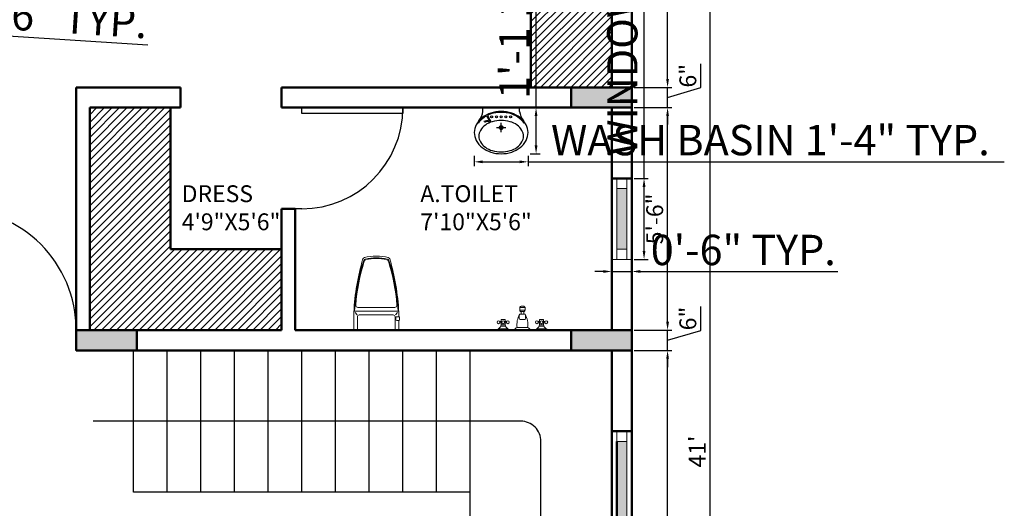
# Model space of a CAD drawing. Units: inches. Extents: x 3064 to 19385, y 846 to 15425.
# Tile 74 of 108: x 6629 to 6922, y 1725 to 1870. Entities that reach past the tile are written whole.
import ezdxf

# ---------------------------------------------------------------- set-up
doc = ezdxf.new("R2010")
doc.units = ezdxf.units.IN
for name, color, linetype, lineweight in [('A-ANNO-DIMS', 2, 'Continuous', 18), ('A-AREA-IDEN', 3, 'Continuous', 18), ('A-COLS', 1, 'Continuous', 35), ('A-DOOR', 3, 'Continuous', 25), ('A-FLOR-FIXT', 9, 'Continuous', 18), ('A-FLOR-STRS', 2, 'Continuous', 25), ('A-FURN-PATT', 252, 'Continuous', 13), ('A-GLAZ', 4, 'Continuous', 18), ('A-WALL', 7, 'Continuous', 50)]:
    doc.layers.add(name, color=color, linetype=linetype, lineweight=lineweight)
doc.layers.add('THIET-BI', color=21, linetype='Continuous')
doc.styles.get("Standard").update_dxf_attribs({"font": 'arial.ttf'})
doc.dimstyles.new('ISO-25', dxfattribs={"dimtxt": 9, "dimasz": 2.5, "dimexe": 1.25, "dimexo": 0.625, "dimtad": 1, "dimdec": 1, "dimlunit": 3, "dimtxsty": 'Standard', "dimcen": 2.5, "dimadec": 0, "dimazin": 0, "dimtfac": 1, "dimtdec": 1, "dimtmove": 0, "dimatfit": 3, "dimfxl": 1, "dimarcsym": 0})
pattern_1 = [(45, (2126.5405, 591.649), (-1.122532, 1.122532), [])]

# ---------------------------------------------------------------- blocks, each defined once
blk = doc.blocks.new('*U3')
for p, q in [((0, 0), (0, -6)), ((36, 0), (36, -6))]:
    blk.add_line(p, q)
blk.add_lwpolyline([(0, 0), (0, 36), (1.75, 36), (1.75, 0)], close=True)
blk.add_arc((0, 0), 36, 0, 90)
blk = doc.blocks.new('*U4')
for p, q in [((0, 0), (0, -6)), ((30, 0), (30, -6))]:
    blk.add_line(p, q)
blk.add_lwpolyline([(0, 0), (0, 30), (1.75, 30), (1.75, 0)], close=True)
blk.add_arc((0, 0), 30, 0, 90)
blk = doc.blocks.new('A$C430D11A0')
at = {"layer": 'THIET-BI'}
for p, q in [((90, 445), (90, 485)), ((475, 485), (90, 485)), ((475, 483), (90, 483)), ((475, 445), (475, 485)), ((129, 398), (158, 344)), ((138, 403), (176, 332)), ((282, 226), (282, 325)), ((233, 275), (332, 275))]:
    blk.add_line(p, q, dxfattribs=at)
for points in [[(565, 223, 0.121635), (545, 305, 0.10526), (482, 380, 0.088175), (393, 427, 0.079002), (282, 445, 0.079002), (172, 427, 0.088175), (83, 380, 0.10526), (20, 305, 0.121635), (0, 223, 0.121635), (20, 140, 0.10526), (83, 65, 0.088175), (172, 18, 0.079002), (282, 0, 0.079002), (393, 18, 0.088175), (482, 65, 0.10526), (545, 140, 0.121635)], [(517, 185, 0.134042), (501, 245, 0.106817), (449, 302, 0.082468), (376, 337, 0.070874), (282, 350, 0.070874), (189, 337, 0.082468), (116, 302, 0.106817), (64, 245, 0.134042), (47, 185, 0.134042), (64, 125, 0.106817), (116, 68, 0.082468), (189, 33, 0.070874), (282, 20, 0.070874), (376, 33, 0.082468), (449, 68, 0.106817), (501, 125, 0.134042)]]:
    blk.add_lwpolyline(points, format="xyb", close=True, dxfattribs=at)
for points in [[(523, 322, 0.07708), (476, 372, 0.088175), (390, 418, 0.079002), (282, 435, 0.079002), (175, 418, 0.035427), (138, 403, 0.07708)], [(129, 398, 0.043566), (89, 372, 0.07708), (42, 322, 0.041486)]]:
    blk.add_lwpolyline(points, format="xyb", dxfattribs=at)
for centre, radius in [((182, 388), 10.5), ((232, 388), 10.5), ((282, 388), 10.5), ((332, 388), 10.5), ((382, 388), 10.5), ((282, 275), 20), ((282, 275), 15)]:
    blk.add_circle(centre, radius, dxfattribs=at)
for centre, radius, start, end in [((-104, 469), 195, 320.8253, 352.9557), ((669, 469), 195, 187.0443, 219.1747), ((136, 285), 62.9, 69.643, 123.4774), ((136, 285), 52.9, 55.2455, 123.4774)]:
    blk.add_arc(centre, radius, start, end, dxfattribs=at)
blk = doc.blocks.new('WC-P05')
for p, q in [((-202, 532), (-202, 439)), ((-192, 542), (263, 542)), ((-163, 542), (-163, 401)), ((234, 542), (234, 401)), ((273, 532), (273, 352)), ((-210, 430), (-210, 409)), ((-201, 439), (-180, 439)), ((-171, 430), (-171, 409)), ((-202, 400), (-202, 352)), ((-201, 400), (-180, 400)), ((-192, 342), (263, 342)), ((-167, 379), (-188, 357)), ((-143, 381), (214, 381)), ((237, 379), (258, 357)), ((-159, 303), (229, 303))]:
    blk.add_line(p, q)
blk.add_lwpolyline([(-91, -222, 0.114547), (161, -222, 0.114547)], format="xyb")
for centre, radius, start, end in [((-192, 532), 10, 90, 180), ((263, 532), 10, 0, 90), ((-201, 430), 9, 90, 180), ((-180, 430), 9, 0, 90), ((-201, 409), 9, 180, 270), ((2309, 492), 2515, 183.2067, 196.1242), ((-192, 352), 10, 180, 270), ((1906, 447), 2103, 182.8743, 197.6554), ((-180, 409), 9, 270, 0), ((-143, 401), 20, 180, 270), ((-1836, 447), 2103, 342.3446, 357.1257), ((-2239, 492), 2515, 343.8727, 356.7933), ((214, 401), 20, 270, 0), ((263, 352), 10, 270, 0), ((-159, 280), 22.5, 90, 184.6246), ((1906, 447), 2095, 184.6245, 197.5277), ((-1836, 447), 2095, 342.464, 355.3754), ((229, 280), 22.5, 355.3754, 90), ((-86, -200), 22.5, 196.1242, 256.8994), ((-76, -184), 22.5, 197.6554, 257.5059), ((-70, -177), 22.5, 197.5277, 258.1005), ((35, 318), 536, 257.5059, 282.4941), ((36, 324), 535, 258.1005, 281.7373), ((140, -177), 22.5, 281.7373, 342.464), ((146, -184), 22.5, 282.4941, 342.3446), ((156, -200), 22.5, 283.0378, 343.8727)]:
    blk.add_arc(centre, radius, start, end)
blk = doc.blocks.new('Faucet - Bathroom front')
for p, q in [((-0.5, 4.25), (0.5, 4.25)), ((0.5, 3.75), (-0.5, 3.75)), ((-0.5, 3), (0.5, 3)), ((0.5, 2), (-0.5, 2)), ((-0.25, 3), (-0.25, 3.5)), ((0.25, 3.5), (0.25, 3)), ((-5, 0), (-2.25, 0)), ((-4.5087, 0.25), (-2.7408, 0.25)), ((-4, 1.625), (-4.25, 1.625)), ((-4, 1.375), (-4.25, 1.375)), ((-3.1442, 0.75), (-4.0979, 0.75)), ((-3.25, 1.625), (-3, 1.625)), ((-3.25, 1.375), (-3, 1.375)), ((-1.5, 0), (1.5, 0)), ((-1, 0.5), (1, 0.5)), ((2.25, 0), (5, 0)), ((2.7413, 0.25), (4.5092, 0.25)), ((3.25, 1.625), (3, 1.625)), ((3.25, 1.375), (3, 1.375)), ((4.1058, 0.75), (3.1521, 0.75)), ((4, 1.625), (4.25, 1.625)), ((4, 1.375), (4.25, 1.375))]:
    blk.add_line(p, q)
for points in [[(-0.5, 3.75), (-0.5, 4.25)], [(-0.25, 4.5), (0.25, 4.5)], [(0.5, 4.25), (0.5, 3.75)], [(0.25, 3.5), (-0.25, 3.5)]]:
    blk.add_lwpolyline(points)
for points in [[(-4, 1), (-4, 2), (-3.25, 2), (-3.25, 1)], [(3.25, 1), (3.25, 2), (4, 2), (4, 1)]]:
    blk.add_lwpolyline(points, close=True)
for centre in [(-4.5, 1.5), (-3.625, 1.5), (-2.75, 1.5), (2.75, 1.5), (3.625, 1.5), (4.5, 1.5)]:
    blk.add_circle(centre, 0.2795)
for centre, radius, start, end in [((-0.2575, 4.2575), 0.2426, 88.22243, 181.7776), ((-0.2575, 3.7425), 0.2426, 178.2224, 271.7776), ((0.2575, 4.2575), 0.2426, 358.2224, 91.77757), ((0.2575, 3.7425), 0.2426, 268.2224, 1.777565), ((3, 1), 4.0311, 150.2551, 187.125), ((0.6413, 2.5), 1.246, 156.3417, 203.6583), ((-3, 1), 4.0311, 352.875, 29.74488), ((-0.6413, 2.5), 1.246, 336.3417, 23.65835), ((-5.375, 1.375), 1.4252, 285.2551, 344.7449), ((-1.875, 1.375), 1.4252, 195.2551, 254.7449), ((-0.7962, -0.2038), 0.7327, 106.1502, 163.8498), ((0.7962, -0.2038), 0.7327, 16.1502, 73.84979), ((1.875, 1.375), 1.4252, 285.2551, 344.7449), ((5.375, 1.375), 1.4252, 195.2551, 254.7449)]:
    blk.add_arc(centre, radius, start, end)
blk = doc.blocks.new('*D363')
at = {"layer": 'A-ANNO-DIMS', "color": 0, "lineweight": -2, "transparency": 16777216}
for p, q in [((6811.66, 1771.99), (6822.87, 1771.99)), ((6821.62, 1576.49), (6821.62, 1769.49)), ((6805.66, 1573.99), (6822.87, 1573.99))]:
    blk.add_line(p, q, dxfattribs=at)
at = {"layer": 'A-ANNO-DIMS', "color": 0, "transparency": 16777216}
for points in [[(6821.2, 1769.49), (6822.03, 1769.49), (6821.62, 1771.99)], [(6821.2, 1576.49), (6822.03, 1576.49), (6821.62, 1573.99)]]:
    blk.add_solid(points, dxfattribs=at)
at = {"layer": 'Defpoints', "color": 0, "transparency": 16777216}
for p in [(6811.03, 1771.99), (6821.62, 1771.99), (6805.03, 1573.99)]:
    blk.add_point(p, dxfattribs=at)
at = {"layer": 'A-ANNO-DIMS', "color": 0, "transparency": 16777216, "insert": (6818.44, 1672.99), "char_height": 5, "attachment_point": 5, "rotation": 90}
blk.add_mtext('16\'-6"', dxfattribs=at)
blk = doc.blocks.new('*D364')
at = {"layer": 'A-ANNO-DIMS', "color": 0, "lineweight": -2, "transparency": 16777216}
for p, q in [((6831.46, 1777.94), (6831.46, 1784.97)), ((6821.62, 1780.49), (6821.62, 1782.99)), ((6811.66, 1777.99), (6822.87, 1777.99)), ((6821.62, 1771.99), (6821.62, 1777.99)), ((6821.62, 1771.99), (6821.62, 1777.99)), ((6821.62, 1774.99), (6831.46, 1777.94)), ((6811.66, 1771.99), (6822.87, 1771.99)), ((6821.62, 1769.49), (6821.62, 1766.99))]:
    blk.add_line(p, q, dxfattribs=at)
at = {"layer": 'A-ANNO-DIMS', "color": 0, "transparency": 16777216}
for points in [[(6821.2, 1780.49), (6822.03, 1780.49), (6821.62, 1777.99)], [(6821.2, 1769.49), (6822.03, 1769.49), (6821.62, 1771.99)]]:
    blk.add_solid(points, dxfattribs=at)
at = {"layer": 'Defpoints', "color": 0, "transparency": 16777216}
for p in [(6811.03, 1777.99), (6821.62, 1777.99), (6811.03, 1771.99)]:
    blk.add_point(p, dxfattribs=at)
at = {"layer": 'A-ANNO-DIMS', "color": 0, "transparency": 16777216, "insert": (6828.28, 1781.45), "char_height": 5, "attachment_point": 5, "rotation": 90}
blk.add_mtext('6"', dxfattribs=at)
blk = doc.blocks.new('*D365')
at = {"layer": 'A-ANNO-DIMS', "color": 0, "lineweight": -2, "transparency": 16777216}
for p, q in [((6811.66, 1843.99), (6822.87, 1843.99)), ((6821.62, 1780.49), (6821.62, 1841.49)), ((6811.66, 1777.99), (6822.87, 1777.99))]:
    blk.add_line(p, q, dxfattribs=at)
at = {"layer": 'A-ANNO-DIMS', "color": 0, "transparency": 16777216}
for points in [[(6821.2, 1841.49), (6822.03, 1841.49), (6821.62, 1843.99)], [(6821.2, 1780.49), (6822.03, 1780.49), (6821.62, 1777.99)]]:
    blk.add_solid(points, dxfattribs=at)
at = {"layer": 'Defpoints', "color": 0, "transparency": 16777216}
for p in [(6811.03, 1843.99), (6821.62, 1843.99), (6811.03, 1777.99)]:
    blk.add_point(p, dxfattribs=at)
at = {"layer": 'A-ANNO-DIMS', "color": 0, "transparency": 16777216, "insert": (6818.44, 1810.99), "char_height": 5, "attachment_point": 5, "rotation": 90}
blk.add_mtext('5\'-6"', dxfattribs=at)
blk = doc.blocks.new('*D366')
at = {"layer": 'A-ANNO-DIMS', "color": 0, "lineweight": -2, "transparency": 16777216}
for p, q in [((6831.46, 1849.94), (6831.46, 1856.97)), ((6821.62, 1852.49), (6821.62, 1854.99)), ((6811.66, 1849.99), (6822.87, 1849.99)), ((6821.62, 1843.99), (6821.62, 1849.99)), ((6821.62, 1843.99), (6821.62, 1849.99)), ((6821.62, 1846.99), (6831.46, 1849.94)), ((6811.66, 1843.99), (6822.87, 1843.99)), ((6821.62, 1841.49), (6821.62, 1838.99))]:
    blk.add_line(p, q, dxfattribs=at)
at = {"layer": 'A-ANNO-DIMS', "color": 0, "transparency": 16777216}
for points in [[(6821.2, 1852.49), (6822.03, 1852.49), (6821.62, 1849.99)], [(6821.2, 1841.49), (6822.03, 1841.49), (6821.62, 1843.99)]]:
    blk.add_solid(points, dxfattribs=at)
at = {"layer": 'Defpoints', "color": 0, "transparency": 16777216}
for p in [(6811.03, 1849.99), (6821.62, 1849.99), (6811.03, 1843.99)]:
    blk.add_point(p, dxfattribs=at)
at = {"layer": 'A-ANNO-DIMS', "color": 0, "transparency": 16777216, "insert": (6828.28, 1853.45), "char_height": 5, "attachment_point": 5, "rotation": 90}
blk.add_mtext('6"', dxfattribs=at)
blk = doc.blocks.new('*D346')
at = {"layer": 'A-ANNO-DIMS', "color": 0, "lineweight": -2, "transparency": 16777216}
for p, q in [((6805.66, 1981.99), (6822.87, 1981.99)), ((6821.62, 1852.49), (6821.62, 1979.49)), ((6811.66, 1849.99), (6822.87, 1849.99))]:
    blk.add_line(p, q, dxfattribs=at)
at = {"layer": 'A-ANNO-DIMS', "color": 0, "transparency": 16777216}
for points in [[(6821.2, 1979.49), (6822.03, 1979.49), (6821.62, 1981.99)], [(6821.2, 1852.49), (6822.03, 1852.49), (6821.62, 1849.99)]]:
    blk.add_solid(points, dxfattribs=at)
at = {"layer": 'Defpoints', "color": 0, "transparency": 16777216}
for p in [(6805.03, 1981.99), (6821.62, 1981.99), (6811.03, 1849.99)]:
    blk.add_point(p, dxfattribs=at)
at = {"layer": 'A-ANNO-DIMS', "color": 0, "transparency": 16777216, "insert": (6818.48, 1915.99), "char_height": 5, "attachment_point": 5, "rotation": 90}
blk.add_mtext("11'", dxfattribs=at)
blk = doc.blocks.new('*D348')
at = {"layer": 'A-ANNO-DIMS', "color": 0, "lineweight": -2, "transparency": 16777216}
for p, q in [((6811.66, 1987.99), (6835.44, 1987.99)), ((6834.19, 1985.49), (6834.19, 1498.49)), ((6811.66, 1495.99), (6835.44, 1495.99))]:
    blk.add_line(p, q, dxfattribs=at)
at = {"layer": 'A-ANNO-DIMS', "color": 0, "transparency": 16777216}
for points in [[(6833.77, 1985.49), (6834.6, 1985.49), (6834.19, 1987.99)], [(6833.77, 1498.49), (6834.6, 1498.49), (6834.19, 1495.99)]]:
    blk.add_solid(points, dxfattribs=at)
at = {"layer": 'Defpoints', "color": 0, "transparency": 16777216}
for p in [(6811.03, 1987.99), (6811.03, 1495.99), (6834.19, 1495.99)]:
    blk.add_point(p, dxfattribs=at)
at = {"layer": 'A-ANNO-DIMS', "color": 0, "transparency": 16777216, "insert": (6831.05, 1741.99), "char_height": 5, "attachment_point": 5, "rotation": 90}
blk.add_mtext("41'", dxfattribs=at)
blk = doc.blocks.new('WIN-1800-PAIR')
h = blk.add_hatch(color=256)
h.dxf.hatch_style = 1
h.paths.add_polyline_path([(0, 0), (3, 0), (3, 70.5), (0, 70.5)])
h.paths.add_polyline_path([(3, 144), (0, 144), (0, 73.5), (3, 73.5)])
blk.add_line((3, 144), (3, 73.5))
blk.add_lwpolyline([(3, 144), (0, 144), (0, 147), (3, 147)], close=True)
blk = doc.blocks.new('WIN-600-B')
h = blk.add_hatch(color=256)
h.dxf.hatch_style = 1
h.paths.add_polyline_path([(4.5, 21), (1.5, 21), (1.5, 3), (4.5, 3)])
for p, q in [((1.5, 21), (1.5, 3)), ((4.5, 21), (4.5, 3)), ((0, 0), (6, 0))]:
    blk.add_line(p, q)
for points in [[(4.5, 21), (1.5, 21), (1.5, 24), (4.5, 24)], [(4.5, 0), (1.5, 0), (1.5, 3), (4.5, 3)]]:
    blk.add_lwpolyline(points, close=True)
blk = doc.blocks.new('*D403')
at = {"layer": 'A-ANNO-DIMS', "color": 0, "lineweight": -2, "transparency": 16777216}
for p, q in [((6764.24, 1829.68), (6764.24, 1826.66)), ((6766.74, 1827.91), (6777.68, 1827.91)), ((6780.18, 1829.68), (6780.18, 1826.66)), ((6780.18, 1827.91), (6921.6, 1827.91))]:
    blk.add_line(p, q, dxfattribs=at)
at = {"layer": 'A-ANNO-DIMS', "color": 0, "transparency": 16777216}
for points in [[(6766.74, 1828.33), (6766.74, 1827.49), (6764.24, 1827.91)], [(6777.68, 1828.33), (6777.68, 1827.49), (6780.18, 1827.91)]]:
    blk.add_solid(points, dxfattribs=at)
at = {"layer": 'Defpoints', "color": 0, "transparency": 16777216}
for p in [(6764.24, 1830.3), (6780.18, 1830.3), (6780.18, 1827.91)]:
    blk.add_point(p, dxfattribs=at)
at = {"layer": 'A-ANNO-DIMS', "color": 0, "transparency": 16777216, "insert": (6852.14, 1833.19), "char_height": 9, "attachment_point": 5}
blk.add_mtext('WASH BASIN 1\'-4" TYP.', dxfattribs=at)
blk = doc.blocks.new('*D404')
at = {"layer": 'A-ANNO-DIMS', "color": 0, "lineweight": -2, "transparency": 16777216}
for p, q in [((6782.57, 1843.99), (6782.57, 1922.72)), ((6780.81, 1843.99), (6783.82, 1843.99)), ((6782.57, 1832.8), (6782.57, 1841.49)), ((6780.81, 1830.3), (6783.82, 1830.3))]:
    blk.add_line(p, q, dxfattribs=at)
at = {"layer": 'A-ANNO-DIMS', "color": 0, "transparency": 16777216}
for points in [[(6782.16, 1841.49), (6782.99, 1841.49), (6782.57, 1843.99)], [(6782.16, 1832.8), (6782.99, 1832.8), (6782.57, 1830.3)]]:
    blk.add_solid(points, dxfattribs=at)
at = {"layer": 'Defpoints', "color": 0, "transparency": 16777216}
for p in [(6780.18, 1843.99), (6782.57, 1843.99), (6780.18, 1830.3)]:
    blk.add_point(p, dxfattribs=at)
at = {"layer": 'A-ANNO-DIMS', "color": 0, "transparency": 16777216, "insert": (6777.29, 1884.61), "char_height": 9, "attachment_point": 5, "rotation": 90}
blk.add_mtext('1\'-1 1/2" TYP.', dxfattribs=at)
blk = doc.blocks.new('*D434')
at = {"layer": 'A-ANNO-DIMS', "color": 0, "lineweight": -2, "transparency": 16777216}
for p, q in [((6601, 1876.66), (6600.29, 1865.71)), ((6606.99, 1876.27), (6606.28, 1865.32)), ((6597.88, 1867.12), (6595.38, 1867.28)), ((6600.37, 1866.95), (6606.36, 1866.56)), ((6608.85, 1866.4), (6667.34, 1862.59))]:
    blk.add_line(p, q, dxfattribs=at)
at = {"layer": 'A-ANNO-DIMS', "color": 0, "transparency": 16777216}
for points in [[(6597.9, 1867.53), (6597.85, 1866.7), (6600.37, 1866.95)], [(6608.88, 1866.82), (6608.83, 1865.99), (6606.36, 1866.56)]]:
    blk.add_solid(points, dxfattribs=at)
at = {"layer": 'Defpoints', "color": 0, "transparency": 16777216}
for p in [(6601.04, 1877.28), (6607.03, 1876.89), (6606.36, 1866.56)]:
    blk.add_point(p, dxfattribs=at)
at = {"layer": 'A-ANNO-DIMS', "color": 0, "transparency": 16777216, "insert": (6639.68, 1869.62), "char_height": 9, "attachment_point": 5, "rotation": 356.2748}
blk.add_mtext('0\'-6" TYP.', dxfattribs=at)
blk = doc.blocks.new('*D441')
at = {"layer": 'A-ANNO-DIMS', "color": 0, "lineweight": -2, "transparency": 16777216}
for p, q in [((6814.63, 1822.99), (6814.63, 1989.54)), ((6811.66, 1822.99), (6815.88, 1822.99)), ((6814.63, 1801.49), (6814.63, 1820.49)), ((6811.66, 1798.99), (6815.88, 1798.99))]:
    blk.add_line(p, q, dxfattribs=at)
at = {"layer": 'A-ANNO-DIMS', "color": 0, "transparency": 16777216}
for points in [[(6814.22, 1820.49), (6815.05, 1820.49), (6814.63, 1822.99)], [(6814.22, 1801.49), (6815.05, 1801.49), (6814.63, 1798.99)]]:
    blk.add_solid(points, dxfattribs=at)
at = {"layer": 'Defpoints', "color": 0, "transparency": 16777216}
for p in [(6811.03, 1822.99), (6814.63, 1822.99), (6811.03, 1798.99)]:
    blk.add_point(p, dxfattribs=at)
at = {"layer": 'A-ANNO-DIMS', "color": 0, "transparency": 16777216, "insert": (6809.35, 1907.51), "char_height": 9, "attachment_point": 5, "rotation": 90}
blk.add_mtext('WINDOW W600-B 2\'-0" TYP.', dxfattribs=at)
blk = doc.blocks.new('*D442')
at = {"layer": 'A-ANNO-DIMS', "color": 0, "lineweight": -2, "transparency": 16777216}
for p, q in [((6805.03, 1798.36), (6805.03, 1794.14)), ((6811.03, 1798.36), (6811.03, 1794.14)), ((6802.53, 1795.39), (6800.03, 1795.39)), ((6805.03, 1795.39), (6811.03, 1795.39)), ((6813.53, 1795.39), (6872.14, 1795.39))]:
    blk.add_line(p, q, dxfattribs=at)
at = {"layer": 'A-ANNO-DIMS', "color": 0, "transparency": 16777216}
for points in [[(6802.53, 1795.81), (6802.53, 1794.97), (6805.03, 1795.39)], [(6813.53, 1795.81), (6813.53, 1794.97), (6811.03, 1795.39)]]:
    blk.add_solid(points, dxfattribs=at)
at = {"layer": 'Defpoints', "color": 0, "transparency": 16777216}
for p in [(6805.03, 1798.99), (6811.03, 1798.99), (6811.03, 1795.39)]:
    blk.add_point(p, dxfattribs=at)
at = {"layer": 'A-ANNO-DIMS', "color": 0, "transparency": 16777216, "insert": (6844.09, 1800.61), "char_height": 9, "attachment_point": 5}
blk.add_mtext('0\'-6" TYP.', dxfattribs=at)

msp = doc.modelspace()

# ---------------------------------------------------------------- hatches: boundary and pattern name
at = {"layer": 'A-COLS'}
h = msp.add_hatch(color=256, dxfattribs=at)
h.dxf.hatch_style = 1
h.paths.add_polyline_path([(6811.03, 1843.99), (6811.03, 1849.99), (6793.03, 1849.99), (6793.03, 1843.99)])
h = msp.add_hatch(color=256, dxfattribs=at)
h.dxf.hatch_style = 1
h.paths.add_polyline_path([(6664.03, 1771.99), (6664.03, 1777.99), (6646.03, 1777.99), (6646.03, 1771.99)])
h = msp.add_hatch(color=256, dxfattribs=at)
h.dxf.hatch_style = 1
h.paths.add_polyline_path([(6811.03, 1771.99), (6811.03, 1777.99), (6793.03, 1777.99), (6793.03, 1771.99)])
at = {"layer": 'A-FURN-PATT'}
h = msp.add_hatch(dxfattribs=at)
h.set_pattern_fill('ANSI31', color=256, scale=0.5)
h.set_pattern_definition(pattern_1)
h.paths.add_polyline_path([(6781.03, 1849.99), (6805.03, 1849.99), (6805.03, 1981.99), (6781.03, 1981.99)])
h = msp.add_hatch(dxfattribs=at)
h.set_pattern_fill('ANSI31', color=256, scale=0.5)
h.set_pattern_definition(pattern_1)
h.paths.add_polyline_path([(6674.03, 1801.99), (6674.03, 1843.99), (6650.03, 1843.99), (6650.03, 1777.99), (6664.03, 1777.99), (6707.03, 1777.99), (6707.03, 1801.99)])

# ---------------------------------------------------------------- linework, layer by layer
at = {"layer": 'A-FLOR-STRS'}
for p, q in [((6663.03, 1729.99), (6663.03, 1771.99)), ((6673.03, 1729.99), (6673.03, 1771.99)), ((6683.03, 1729.99), (6683.03, 1771.99)), ((6693.03, 1729.99), (6693.03, 1771.99)), ((6703.03, 1729.99), (6703.03, 1771.99)), ((6713.03, 1729.99), (6713.03, 1771.99)), ((6723.03, 1729.99), (6723.03, 1771.99)), ((6733.03, 1729.99), (6733.03, 1771.99)), ((6743.03, 1729.99), (6743.03, 1771.99)), ((6753.03, 1729.99), (6753.03, 1771.99)), ((6763.03, 1615.99), (6763.03, 1771.99)), ((6763.03, 1729.99), (6663.03, 1729.99))]:
    msp.add_line(p, q, dxfattribs=at)
msp.add_lwpolyline([(6670.52, 1594.99), (6778.03, 1594.99, 0.414214), (6784.03, 1600.99), (6784.03, 1744.99, 0.414214), (6778.03, 1750.99), (6651.03, 1750.99)], format="xyb", dxfattribs=at)
at = {"layer": 'A-WALL'}
for p, q in [((6811.03, 1495.99), (6811.03, 1987.99)), ((6781.03, 1849.99), (6781.03, 1981.99)), ((6805.03, 1849.99), (6805.03, 1981.99)), ((6677.03, 1849.99), (6646.03, 1849.99)), ((6646.03, 1849.99), (6646.03, 1771.99)), ((6677.03, 1849.99), (6677.03, 1843.99)), ((6805.03, 1849.99), (6707.03, 1849.99)), ((6707.03, 1849.99), (6707.03, 1843.99)), ((6677.03, 1843.99), (6650.03, 1843.99)), ((6650.03, 1843.99), (6650.03, 1777.99)), ((6674.03, 1843.99), (6674.03, 1801.99)), ((6805.03, 1843.99), (6707.03, 1843.99)), ((6805.03, 1777.99), (6805.03, 1843.99)), ((6805.03, 1822.99), (6811.03, 1822.99)), ((6711.03, 1813.99), (6707.03, 1813.99)), ((6707.03, 1813.99), (6707.03, 1777.99)), ((6711.03, 1777.99), (6711.03, 1813.99)), ((6707.03, 1801.99), (6674.03, 1801.99)), ((6707.03, 1777.99), (6650.03, 1777.99)), ((6805.03, 1777.99), (6711.03, 1777.99)), ((6805.03, 1771.99), (6646.03, 1771.99)), ((6805.03, 1573.99), (6805.03, 1771.99)), ((6811.03, 1747.99), (6805.03, 1747.99)), ((6806.53, 1744.99), (6806.53, 1674.49))]:
    msp.add_line(p, q, dxfattribs=at)
for points in [[(6811.03, 1849.99), (6793.03, 1849.99), (6793.03, 1843.99), (6811.03, 1843.99)], [(6664.03, 1777.99), (6646.03, 1777.99), (6646.03, 1771.99), (6664.03, 1771.99)], [(6811.03, 1777.99), (6793.03, 1777.99), (6793.03, 1771.99), (6811.03, 1771.99)]]:
    msp.add_lwpolyline(points, close=True, dxfattribs=at)

# ---------------------------------------------------------------- block references
at = {"layer": 'A-DOOR', "rotation": 270}
msp.add_blockref('*U4', (6713.03, 1843.99), dxfattribs=at)
at = {"layer": 'A-DOOR'}
msp.add_blockref('*U3', (6610.03, 1777.99), dxfattribs=at)
at = {"layer": 'A-FLOR-FIXT'}
for name, p, xscale, yscale, zscale in [('A$C430D11A0', (6764.24, 1830.3), 0.0282220760332506, 0.0282220760332506, 0.0282220760332506), ('Faucet - Bathroom front', (6778.5, 1777.99), 1.573166238287219, 1.573166238287219, 1.573166238287219)]:
    msp.add_blockref(name, p, dxfattribs=dict(at, xscale=xscale, yscale=yscale, zscale=zscale))
at = {"layer": 'A-FLOR-FIXT', "xscale": 0.0282220760332506, "yscale": 0.0282220760332506, "zscale": 0.0282220760332506, "rotation": 180}
msp.add_blockref('WC-P05', (6736.13, 1793.28), dxfattribs=at)
at = {"layer": 'A-GLAZ'}
for name, p in [('WIN-600-B', (6805.03, 1798.99)), ('WIN-1800-PAIR', (6806.53, 1600.99))]:
    msp.add_blockref(name, p, dxfattribs=at)

# ---------------------------------------------------------------- texts
at = {"layer": 'A-AREA-IDEN', "char_height": 5, "attachment_point": 1}
for s, insert in [('DRESS\\P4\'9"X5\'6"', (6677.36, 1820.96)), ('A.TOILET\\P7\'10"X5\'6"', (6748.2, 1820.96))]:
    msp.add_mtext_dynamic_manual_height_columns(s, width=67.5924, gutter_width=12.5, heights=[0], dxfattribs=dict(at, insert=insert))

# ---------------------------------------------------------------- dimensions: what is measured, and where the dimension line sits
at = {"layer": 'A-ANNO-DIMS'}
for base, p1, p2, angle, text, picture, middle in [((6814.63, 1822.99), (6811.03, 1798.99), (6811.03, 1822.99), 90, 'WINDOW W600-B <> TYP.', '*D441', (6809.35, 1907.51)), ((6782.57, 1843.99), (6780.18, 1830.3), (6780.18, 1843.99), 90, '<> TYP.', '*D404', (6777.29, 1884.61)), ((6606.36, 1866.56), (6601.04, 1877.28), (6607.03, 1876.89), 356.2748, '<> TYP.', '*D434', (6639.68, 1869.62))]:
    dim = msp.add_linear_dim(base=base, p1=p1, p2=p2, angle=angle, text=text, dimstyle='ISO-25', override={"dimdec": 1, "dimrnd": 0, "dimzin": 1, "dimlunit": 4, "dimfrac": 2}, dxfattribs=at)
    dim.commit()
    dim.dimension.update_dxf_attribs({"geometry": picture, "text_midpoint": middle})
for base, p1, p2, override, picture, middle in [((6834.19, 1495.99), (6811.03, 1987.99), (6811.03, 1495.99), {"dimtxt": 5, "dimclrd": 0, "dimclre": 0, "dimclrt": 0}, '*D348', (6831.05, 1741.99)), ((6821.62, 1981.99), (6811.03, 1849.99), (6805.03, 1981.99), {"dimtxt": 5, "dimclrd": 0, "dimclre": 0, "dimclrt": 0, "dimtmove": 1}, '*D346', (6818.48, 1915.99)), ((6821.62, 1849.99), (6811.03, 1843.99), (6811.03, 1849.99), {"dimtxt": 5, "dimclrd": 0, "dimclre": 0, "dimclrt": 0, "dimtmove": 1}, '*D366', (6828.28, 1850.57)), ((6821.62, 1843.99), (6811.03, 1777.99), (6811.03, 1843.99), {"dimtxt": 5, "dimclrd": 0, "dimclre": 0, "dimclrt": 0, "dimtmove": 1}, '*D365', (6818.44, 1810.99)), ((6821.62, 1777.99), (6811.03, 1771.99), (6811.03, 1777.99), {"dimtxt": 5, "dimclrd": 0, "dimclre": 0, "dimclrt": 0, "dimtmove": 1}, '*D364', (6828.28, 1778.57)), ((6821.62, 1771.99), (6805.03, 1573.99), (6811.03, 1771.99), {"dimtxt": 5, "dimclrd": 0, "dimclre": 0, "dimclrt": 0, "dimtmove": 1}, '*D363', (6818.44, 1672.99))]:
    dim = msp.add_linear_dim(base=base, p1=p1, p2=p2, angle=90, dimstyle='ISO-25', override=override, dxfattribs=at)
    dim.commit()
    dim.dimension.update_dxf_attribs({"geometry": picture, "text_midpoint": middle})
for base, p1, p2, text, picture, middle in [((6780.18, 1827.91), (6764.24, 1830.3), (6780.18, 1830.3), 'WASH BASIN <> TYP.', '*D403', (6852.14, 1833.19)), ((6811.03, 1795.39), (6805.03, 1798.99), (6811.03, 1798.99), '<> TYP.', '*D442', (6844.09, 1800.61))]:
    dim = msp.add_linear_dim(base=base, p1=p1, p2=p2, text=text, dimstyle='ISO-25', override={"dimdec": 1, "dimrnd": 0, "dimzin": 1, "dimlunit": 4, "dimfrac": 2}, dxfattribs=at)
    dim.commit()
    dim.dimension.update_dxf_attribs({"geometry": picture, "text_midpoint": middle})

doc.saveas('drawing.dxf')
